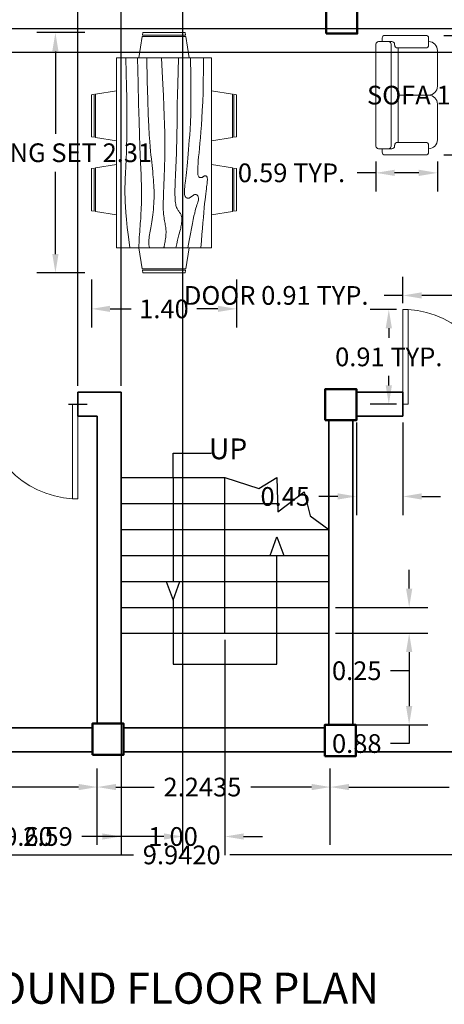
# Model space of a CAD drawing. Units: metres. Extents: x 473.2 to 488.6, y 701.8 to 717.3.
# Tile 2 of 4: x 479.3 to 483.4, y 701.8 to 711.3. Entities that reach past the tile are written whole.
import ezdxf

# ---------------------------------------------------------------- set-up
doc = ezdxf.new("R2010")
doc.units = ezdxf.units.M
doc.header["$PDMODE"] = 32
for name, color, linetype, lineweight in [('A-ANNO-DIMS', 2, 'Continuous', 18), ('A-ANNO-TEXT', 7, 'Continuous', 25), ('A-COLS', 7, 'Continuous', 50), ('A-DOOR', 3, 'Continuous', 18), ('A-FLOR-STRS', 7, 'Continuous', 25), ('A-FURN', 8, 'Continuous', 18), ('A-WALL', 7, 'Continuous', 35)]:
    doc.layers.add(name, color=color, linetype=linetype, lineweight=lineweight)
doc.styles.get("Standard").update_dxf_attribs({"font": 'arial.ttf'})
doc.dimstyles.get("Standard").update_dxf_attribs({"dimtxt": 0.18, "dimasz": 0.18, "dimexe": 0.18, "dimexo": 0.0625, "dimgap": 0.09, "dimtad": 0, "dimtih": 1, "dimtoh": 1, "dimdec": 4, "dimzin": 0, "dimdsep": 46, "dimtxsty": 'Standard', "dimcen": 0.09, "dimadec": 0, "dimazin": 0, "dimtfac": 1, "dimtdec": 4, "dimtofl": 0, "dimtmove": 0, "dimatfit": 3, "dimfxl": 1, "dimtolj": 1, "dimtzin": 0, "dimarcsym": 0})

# ---------------------------------------------------------------- blocks, each defined once
blk = doc.blocks.new('A$C02A636C4')
for p, q in [((1.203, 0.669), (0.097, 0.669)), ((0, 0.572), (0, 0.126)), ((0.068, 0.601), (0.029, 0.601)), ((0.068, 0.64), (0.068, 0.601)), ((0.068, 0.533), (0.068, 0.601)), ((0.068, 0.495), (0.068, 0.543)), ((1.232, 0.64), (1.232, 0.601)), ((1.232, 0.601), (1.271, 0.601)), ((1.232, 0.533), (1.232, 0.601)), ((1.232, 0.495), (1.232, 0.543)), ((1.3, 0.572), (1.3, 0.126)), ((1.203, 0.504), (0.097, 0.504)), ((0.107, 0.466), (0.097, 0.466)), ((0.136, 0.126), (0.136, 0.436)), ((1.164, 0.126), (1.164, 0.436)), ((1.193, 0.466), (1.203, 0.466)), ((1.164, 0.427), (0.136, 0.427)), ((0.65, 0.097), (0.65, 0.427)), ((0.029, 0.097), (0.107, 0.097)), ((0.165, 0), (0.553, 0)), ((0.747, 0), (1.135, 0)), ((1.271, 0.097), (1.193, 0.097))]:
    blk.add_line(p, q)
for centre, radius, start, end in [((0.097, 0.64), 0.0291, 90, 180), ((1.203, 0.64), 0.0291, 0, 90), ((0.029, 0.572), 0.0291, 90, 180), ((1.271, 0.572), 0.0291, 0, 90), ((0.097, 0.533), 0.0291, 180, 270), ((0.097, 0.495), 0.0291, 180, 270), ((0.107, 0.436), 0.0291, 0, 90), ((1.193, 0.436), 0.0291, 90, 180), ((1.203, 0.533), 0.0291, 270, 0), ((1.203, 0.495), 0.0291, 270, 0), ((0.029, 0.126), 0.0291, 180, 270), ((0.107, 0.126), 0.0291, 270, 0), ((1.193, 0.126), 0.0291, 180, 270), ((1.271, 0.126), 0.0291, 270, 0), ((0.165, 0.097), 0.097, 180, 270), ((0.553, 0.097), 0.097, 270, 0), ((0.747, 0.097), 0.097, 180, 270), ((1.135, 0.097), 0.097, 270, 0)]:
    blk.add_arc(centre, radius, start, end)
blk = doc.blocks.new('Dining Set - 36 x 72 in.')
for p, q in [((-22, 27.5), (-22.1562, 26.50042)), ((-5.8416, 26.5), (-22.1534, 26.5)), ((-22, 27.5), (-6, 27.5)), ((-5.8437, 26.49966), (-6, 27.5)), ((6, 27.5), (5.8438, 26.50042)), ((22.1584, 26.5), (5.8466, 26.5)), ((6, 27.5), (22, 27.5)), ((22.1563, 26.49966), (22, 27.5)), ((-22.2343, 26.00059), (-23.4847, 17.99762)), ((-22.2304, 26), (-5.7608, 26)), ((-4.5152, 17.99762), (-5.7655, 25.99926)), ((5.7657, 26.00059), (4.5153, 17.99762)), ((5.7696, 26), (22.2392, 26)), ((23.4848, 17.99762), (22.2345, 25.99926)), ((36, 18), (-36, 18)), ((-36, 18), (-36, -18)), ((36, -18), (36, 18)), ((-45.5, 8), (-44.5004, 8.15617)), ((-45.5, 8), (-45.5, -8)), ((-44.5, -8.15843), (-44.5, 8.15338)), ((-44.0006, 8.23428), (-35.9976, 9.48474)), ((-44, 8.23041), (-44, -8.23915)), ((44.0006, 8.23428), (35.9976, 9.48474)), ((44, 8.23041), (44, -8.23915)), ((44.5, -8.15843), (44.5, 8.15338)), ((45.5, 8), (44.5005, 8.15617)), ((45.5, 8), (45.5, -8)), ((-44.4997, -8.15631), (-45.5, -8)), ((-35.9976, -9.48476), (-43.9993, -8.2345)), ((35.9976, -9.48476), (43.9993, -8.2345)), ((44.4997, -8.15631), (45.5, -8)), ((-36, -18), (36, -18)), ((-22.2343, -26.0006), (-23.4847, -17.99762)), ((-4.5152, -17.99762), (-5.7655, -25.99928)), ((5.7657, -26.0006), (4.5153, -17.99762)), ((23.4848, -17.99762), (22.2345, -25.99928)), ((-22.2304, -26), (-5.7608, -26)), ((5.7696, -26), (22.2392, -26)), ((-22, -27.5), (-22.1562, -26.50044)), ((-5.8416, -26.5), (-22.1534, -26.5)), ((-22, -27.5), (-6, -27.5)), ((-5.8437, -26.49967), (-6, -27.5)), ((6, -27.5), (5.8438, -26.50044)), ((22.1584, -26.5), (5.8466, -26.5)), ((6, -27.5), (22, -27.5)), ((22.1563, -26.49967), (22, -27.5))]:
    blk.add_line(p, q)
for points in [[(-36, 15), (-31.1772, 14.97754), (-26.8079, 14.91406), (-22.8538, 14.81543), (-19.276, 14.6875), (-16.0362, 14.53613), (-13.0957, 14.36718), (-10.4159, 14.18652), (-7.9583, 14), (-5.6904, 13.81315), (-3.6035, 13.63021), (-1.6954, 13.45508), (0.0365, 13.29166), (1.5945, 13.14388), (2.9811, 13.01562), (4.1988, 12.9108), (5.25, 12.83333), (6.1393, 12.78613), (6.8802, 12.76823), (7.4883, 12.77767), (7.9792, 12.8125), (8.3685, 12.87077), (8.6719, 12.95052), (8.9049, 13.0498), (9.0833, 13.16666), (9.2205, 13.29899), (9.3216, 13.44401), (9.3895, 13.59879), (9.4271, 13.76041), (9.4373, 13.92594), (9.4232, 14.09245), (9.3875, 14.257), (9.3333, 14.41666), (9.2638, 14.56917), (9.1836, 14.71484), (9.0975, 14.85465), (9.0104, 14.98958), (8.9272, 15.1206), (8.8529, 15.2487), (8.7922, 15.37483), (8.75, 15.5), (8.7305, 15.62467), (8.7344, 15.74739), (8.7617, 15.86621), (8.8125, 15.97916), (8.8867, 16.08431), (8.9844, 16.17968), (9.1055, 16.26334), (9.25, 16.33333), (9.4189, 16.38802), (9.6172, 16.42708), (9.8506, 16.45052), (10.125, 16.45833), (10.4463, 16.45052), (10.8203, 16.42708), (11.2529, 16.38802), (11.75, 16.33333), (12.3184, 16.26318), (12.9694, 16.17838), (13.7151, 16.07991), (14.5677, 15.96875), (15.5395, 15.84586), (16.6426, 15.71224), (17.8893, 15.56884), (19.2917, 15.41666), (20.859, 15.25667), (22.5879, 15.08984), (24.4721, 14.91715), (26.5052, 14.73958), (28.6809, 14.5581), (30.9929, 14.3737), (33.4347, 14.18733), (36, 14)], [(-36, 10), (-28.9766, 10.14274), (-23.1725, 10.20442), (-18.4241, 10.19775), (-14.5677, 10.13541), (-11.4399, 10.03011), (-8.877, 9.89453), (-6.7154, 9.74137), (-4.7917, 9.58333), (-2.9698, 9.43082), (-1.2246, 9.28515), (0.4415, 9.14534), (2.026, 9.01041), (3.5266, 8.87939), (4.9408, 8.7513), (6.266, 8.62516), (7.5, 8.5), (8.6411, 8.37549), (9.6914, 8.2539), (10.6538, 8.13818), (11.5312, 8.03125), (12.3267, 7.93603), (13.043, 7.85547), (13.6831, 7.79248), (14.25, 7.75), (14.7471, 7.7303), (15.1797, 7.73307), (15.5537, 7.75732), (15.875, 7.80208), (16.1494, 7.86637), (16.3828, 7.94922), (16.5811, 8.04964), (16.75, 8.16666), (16.8944, 8.29915), (17.0143, 8.44531), (17.1089, 8.60319), (17.1771, 8.77083), (17.218, 8.94629), (17.2305, 9.1276), (17.2137, 9.31282), (17.1667, 9.5), (17.0895, 9.6875), (16.987, 9.875), (16.8649, 10.0625), (16.7292, 10.25), (16.5856, 10.4375), (16.4401, 10.625), (16.2985, 10.8125), (16.1667, 11), (16.05, 11.18733), (15.9518, 11.3737), (15.8752, 11.5581), (15.8229, 11.73958), (15.798, 11.91715), (15.8034, 12.08984), (15.842, 12.25667), (15.9167, 12.41666), (16.0295, 12.56836), (16.1784, 12.70833), (16.3605, 12.83268), (16.5729, 12.9375), (16.8127, 13.01888), (17.0768, 13.07291), (17.3625, 13.0957), (17.6667, 13.08333), (17.9894, 13.03312), (18.3418, 12.94726), (18.7382, 12.82918), (19.1927, 12.68229), (19.7195, 12.51001), (20.3327, 12.31575), (21.0465, 12.10294), (21.875, 11.875), (22.8357, 11.63354), (23.959, 11.37304), (25.2786, 11.08618), (26.8282, 10.76562), (28.6414, 10.40405), (30.752, 9.99414), (33.1936, 9.52856), (36, 9)], [(-36, 5.5), (-30.7157, 5.3348), (-26.069, 5.20963), (-21.9946, 5.11767), (-18.4271, 5.05208), (-15.3009, 5.00602), (-12.5508, 4.97265), (-10.1112, 4.94515), (-7.9167, 4.91666), (-5.909, 4.88167), (-4.0586, 4.83984), (-2.3429, 4.79215), (-0.7396, 4.73958), (0.7739, 4.6831), (2.22, 4.6237), (3.6213, 4.56233), (5, 4.5), (6.373, 4.43782), (7.7344, 4.3776), (9.0723, 4.32129), (10.375, 4.27083), (11.6309, 4.22819), (12.8281, 4.19531), (13.9551, 4.17415), (15, 4.16666), (15.954, 4.17448), (16.819, 4.19791), (17.6001, 4.23698), (18.3021, 4.29166), (18.9299, 4.36198), (19.4883, 4.44791), (19.9823, 4.54948), (20.4167, 4.66666), (20.7969, 4.79899), (21.1302, 4.94401), (21.4245, 5.09879), (21.6875, 5.26041), (21.9271, 5.42594), (22.1511, 5.59245), (22.3672, 5.757), (22.5834, 5.91666), (22.8065, 6.06868), (23.0404, 6.21093), (23.2879, 6.34147), (23.5521, 6.45833), (23.8358, 6.55957), (24.142, 6.64323), (24.4735, 6.70735), (24.8334, 6.75), (25.2235, 6.76969), (25.642, 6.76692), (26.0858, 6.74267), (26.5521, 6.69791), (27.0379, 6.63362), (27.5404, 6.55078), (28.0565, 6.45036), (28.5834, 6.33333), (29.1242, 6.19987), (29.7071, 6.04687), (30.3661, 5.87044), (31.1354, 5.66666), (32.0493, 5.43164), (33.142, 5.16146), (34.4475, 4.85221), (36, 4.5)], [(-36, -1), (-30.7915, -0.6591), (-26.0195, -0.38216), (-21.6519, -0.16284), (-17.6563, 0.00521), (-14.0005, 0.12833), (-10.6523, 0.21289), (-7.5796, 0.26522), (-4.75, 0.29166), (-2.134, 0.29793), (0.2878, 0.28711), (2.5317, 0.26163), (4.6146, 0.22396), (6.5529, 0.17651), (8.3633, 0.12174), (10.0623, 0.06209), (11.6667, 0), (13.1899, -0.06201), (14.6341, -0.1211), (15.9982, -0.17432), (17.2813, -0.21875), (18.4823, -0.25147), (19.6003, -0.26953), (20.6343, -0.27002), (21.5834, -0.25), (22.4481, -0.20768), (23.2357, -0.14584), (23.9549, -0.06836), (24.6146, 0.02083), (25.2235, 0.11784), (25.7904, 0.21875), (26.3241, 0.31966), (26.8334, 0.41666), (27.3265, 0.50618), (27.8099, 0.58593), (28.2894, 0.65397), (28.7709, 0.70833), (29.2601, 0.74707), (29.763, 0.76823), (30.2855, 0.76985), (30.8334, 0.75), (31.4088, 0.70784), (31.9994, 0.64713), (32.589, 0.57275), (33.1615, 0.48958), (33.7008, 0.4025), (34.1908, 0.3164), (34.6153, 0.23616), (34.9584, 0.16666), (35.2099, 0.11165), (35.3848, 0.07031), (35.504, 0.04069), (35.5886, 0.02083), (35.6594, 0.00879), (35.7377, 0.0026), (35.8442, 0.00032), (36, 0)], [(-36, -6.5), (-27.1843, -6.31267), (-20.084, -6.1263), (-14.469, -5.9419), (-10.1094, -5.76042), (-6.7752, -5.58285), (-4.2363, -5.41016), (-2.2629, -5.24333), (-0.625, -5.08334), (0.8708, -4.93099), (2.2715, -4.78646), (3.5872, -4.64974), (4.8281, -4.52084), (6.0046, -4.39974), (7.127, -4.28646), (8.2053, -4.18099), (9.25, -4.08334), (10.2705, -3.99382), (11.2734, -3.91407), (12.2647, -3.84603), (13.25, -3.79167), (14.2354, -3.75293), (15.2266, -3.73177), (16.2295, -3.73015), (17.25, -3.75), (18.2912, -3.79248), (19.3451, -3.85547), (20.4009, -3.93604), (21.4479, -4.03125), (22.4754, -4.13819), (23.4727, -4.25391), (24.4289, -4.37549), (25.3334, -4.5), (26.1785, -4.62492), (26.9694, -4.74935), (27.7145, -4.87281), (28.4219, -4.99479), (29.1, -5.11483), (29.7572, -5.23242), (30.4016, -5.34709), (31.0417, -5.45834), (31.6837, -5.56437), (32.3262, -5.65821), (32.9658, -5.73153), (33.599, -5.77604), (34.2224, -5.78345), (34.8327, -5.74545), (35.4264, -5.65373), (36, -5.5)], [(-36, -10), (-26.4022, -9.81299), (-18.4675, -9.62891), (-11.9839, -9.45069), (-6.7396, -9.28125), (-2.5226, -9.12354), (0.8789, -8.98047), (3.6769, -8.85498), (6.0833, -8.75), (8.2767, -8.66765), (10.3021, -8.60677), (12.1712, -8.56543), (13.8958, -8.54167), (15.4876, -8.53353), (16.9583, -8.53907), (18.3197, -8.55632), (19.5834, -8.58334), (20.7616, -8.61841), (21.8685, -8.66081), (22.9188, -8.71004), (23.9271, -8.76563), (24.9081, -8.82707), (25.8763, -8.89388), (26.8465, -8.96558), (27.8334, -9.04167), (28.8474, -9.12118), (29.8828, -9.20117), (30.93, -9.27824), (31.9792, -9.34896), (33.0205, -9.40991), (34.0443, -9.45768), (35.0407, -9.48885), (36, -9.5)], [(-36, -14.5), (-30.0881, -14.33513), (-25.0332, -14.21224), (-20.7312, -14.12647), (-17.0781, -14.07292), (-13.97, -14.04671), (-11.3027, -14.04297), (-8.9724, -14.05681), (-6.875, -14.08334), (-4.9224, -14.11833), (-3.0905, -14.16016), (-1.3709, -14.20785), (0.2448, -14.26042), (1.7647, -14.3169), (3.1973, -14.3763), (4.5507, -14.43767), (5.8333, -14.5), (7.0554, -14.5621), (8.235, -14.62175), (9.3922, -14.67652), (10.5469, -14.72396), (11.7192, -14.76164), (12.929, -14.78711), (14.1965, -14.79794), (15.5417, -14.79167), (16.9933, -14.76424), (18.6152, -14.70508), (20.4804, -14.60197), (22.6615, -14.44271), (25.2312, -14.21509), (28.2624, -13.9069), (31.8277, -13.50594), (36, -13)]]:
    blk.add_lwpolyline(points)
blk = doc.blocks.new('*D18')
at = {"layer": 'A-ANNO-DIMS', "color": 0, "lineweight": -2, "transparency": 16777216}
for p, q in [((475.798, 702.6656), (475.798, 703.4022)), ((485.74, 702.957), (485.74, 703.4022)), ((475.978, 703.2222), (480.3782, 703.2222)), ((485.56, 703.2222), (481.3049, 703.2222))]:
    blk.add_line(p, q, dxfattribs=at)
at = {"layer": 'A-ANNO-DIMS', "color": 0, "transparency": 16777216}
for points in [[(475.978, 703.2522), (475.978, 703.1922), (475.798, 703.2222)], [(485.56, 703.2522), (485.56, 703.1922), (485.74, 703.2222)]]:
    blk.add_solid(points, dxfattribs=at)
at = {"layer": 'Defpoints', "color": 0, "transparency": 16777216}
for p in [(485.74, 703.2222), (485.74, 702.8945), (475.798, 702.6031)]:
    blk.add_point(p, dxfattribs=at)
at = {"layer": 'A-ANNO-DIMS', "color": 0, "transparency": 16777216, "insert": (480.8416, 703.2222), "char_height": 0.18, "width": 1.240263, "attachment_point": 5}
blk.add_mtext('\\A1;9.9420', dxfattribs=at)
blk = doc.blocks.new('*D19')
at = {"layer": 'A-ANNO-DIMS', "color": 0, "lineweight": -2, "transparency": 16777216}
for p, q in [((475.798, 703.4647), (475.798, 704.0553)), ((480.028, 703.6173), (480.028, 704.0553)), ((475.978, 703.8753), (477.468, 703.8753)), ((479.848, 703.8753), (478.4019, 703.8753))]:
    blk.add_line(p, q, dxfattribs=at)
at = {"layer": 'A-ANNO-DIMS', "color": 0, "transparency": 16777216}
for points in [[(475.978, 703.9053), (475.978, 703.8453), (475.798, 703.8753)], [(479.848, 703.9053), (479.848, 703.8453), (480.028, 703.8753)]]:
    blk.add_solid(points, dxfattribs=at)
at = {"layer": 'Defpoints', "color": 0, "transparency": 16777216}
for p in [(480.028, 703.8753), (480.028, 703.5548), (475.798, 703.4022)]:
    blk.add_point(p, dxfattribs=at)
at = {"layer": 'A-ANNO-DIMS', "color": 0, "transparency": 16777216, "insert": (477.9349, 703.8753), "char_height": 0.18, "width": 1.240263, "attachment_point": 5}
blk.add_mtext('\\A1;4.2300', dxfattribs=at)
blk = doc.blocks.new('*D20')
at = {"layer": 'A-ANNO-DIMS', "color": 0, "lineweight": -2, "transparency": 16777216}
for p, q in [((480.028, 703.3187), (480.028, 704.0553)), ((482.2714, 703.601), (482.2714, 704.0553)), ((480.208, 703.8753), (480.5754, 703.8753)), ((482.0914, 703.8753), (481.507, 703.8753))]:
    blk.add_line(p, q, dxfattribs=at)
at = {"layer": 'A-ANNO-DIMS', "color": 0, "transparency": 16777216}
for points in [[(480.208, 703.9053), (480.208, 703.8453), (480.028, 703.8753)], [(482.0914, 703.9053), (482.0914, 703.8453), (482.2714, 703.8753)]]:
    blk.add_solid(points, dxfattribs=at)
at = {"layer": 'Defpoints', "color": 0, "transparency": 16777216}
for p in [(482.2714, 703.8753), (482.2714, 703.5385), (480.028, 703.2562)]:
    blk.add_point(p, dxfattribs=at)
at = {"layer": 'A-ANNO-DIMS', "color": 0, "transparency": 16777216, "insert": (481.0412, 703.8753), "char_height": 0.18, "width": 1.240263, "attachment_point": 5}
blk.add_mtext('\\A1;2.2435', dxfattribs=at)
blk = doc.blocks.new('*D21')
at = {"layer": 'A-ANNO-DIMS', "color": 0, "lineweight": -2, "transparency": 16777216}
for p, q in [((482.2714, 703.3187), (482.2714, 704.0553)), ((485.7234, 703.5853), (485.7234, 704.0553)), ((482.4514, 703.8753), (483.415, 703.8753)), ((485.5434, 703.8753), (484.3415, 703.8753))]:
    blk.add_line(p, q, dxfattribs=at)
at = {"layer": 'A-ANNO-DIMS', "color": 0, "transparency": 16777216}
for points in [[(482.4514, 703.9053), (482.4514, 703.8453), (482.2714, 703.8753)], [(485.5434, 703.9053), (485.5434, 703.8453), (485.7234, 703.8753)]]:
    blk.add_solid(points, dxfattribs=at)
at = {"layer": 'Defpoints', "color": 0, "transparency": 16777216}
for p in [(485.7234, 703.8753), (485.7234, 703.5228), (482.2714, 703.2562)]:
    blk.add_point(p, dxfattribs=at)
at = {"layer": 'A-ANNO-DIMS', "color": 0, "transparency": 16777216, "insert": (483.8782, 703.8753), "char_height": 0.18, "width": 1.240263, "attachment_point": 5}
blk.add_mtext('\\A1;3.4520', dxfattribs=at)
blk = doc.blocks.new('DOOR-SWING-910')
for p, q in [((0, 0), (-0.05, 0)), ((-0.05, 0), (-0.05, -0.91)), ((0, 0), (0, -0.91)), ((0, -0.91), (-0.05, -0.91))]:
    blk.add_line(p, q)
blk.add_arc((0.0015, 0), 0.9115, 180, 266.76381)
blk = doc.blocks.new('COL-SQUARE-300')
blk.add_lwpolyline([(-0.15, -0.15), (0.15, -0.15), (0.15, 0.15), (-0.15, 0.15)], close=True)
blk = doc.blocks.new('*D27')
at = {"layer": 'A-ANNO-DIMS', "color": 0, "lineweight": -2, "transparency": 16777216}
for p, q in [((482.9717, 708.5321), (482.9717, 708.7861)), ((483.8817, 708.5321), (483.8817, 708.7861)), ((482.9717, 708.6061), (482.7917, 708.6061)), ((483.7017, 708.6061), (483.1517, 708.6061))]:
    blk.add_line(p, q, dxfattribs=at)
at = {"layer": 'A-ANNO-DIMS', "color": 0, "transparency": 16777216}
for points in [[(483.1517, 708.6361), (483.1517, 708.5761), (482.9717, 708.6061)], [(483.7017, 708.6361), (483.7017, 708.5761), (483.8817, 708.6061)]]:
    blk.add_solid(points, dxfattribs=at)
at = {"layer": 'Defpoints', "color": 0, "transparency": 16777216}
for p in [(482.9717, 708.6061), (482.9717, 708.4696), (483.8817, 708.4696)]:
    blk.add_point(p, dxfattribs=at)
at = {"layer": 'A-ANNO-DIMS', "color": 0, "transparency": 16777216, "insert": (481.7511, 708.6061), "char_height": 0.18, "attachment_point": 5}
blk.add_mtext('\\A1;DOOR 0.91 TYP.', dxfattribs=at)
blk = doc.blocks.new('*D28')
at = {"layer": 'A-ANNO-DIMS', "color": 0, "lineweight": -2, "transparency": 16777216}
for p, q in [((482.9092, 708.4696), (482.6552, 708.4696)), ((482.8352, 708.2896), (482.8352, 708.1965)), ((482.8352, 707.7396), (482.8352, 707.8327)), ((482.9092, 707.5596), (482.6552, 707.5596))]:
    blk.add_line(p, q, dxfattribs=at)
at = {"layer": 'A-ANNO-DIMS', "color": 0, "transparency": 16777216}
for points in [[(482.8052, 708.2896), (482.8652, 708.2896), (482.8352, 708.4696)], [(482.8052, 707.7396), (482.8652, 707.7396), (482.8352, 707.5596)]]:
    blk.add_solid(points, dxfattribs=at)
at = {"layer": 'Defpoints', "color": 0, "transparency": 16777216}
for p in [(482.9717, 708.4696), (482.8352, 707.5596), (482.9717, 707.5596)]:
    blk.add_point(p, dxfattribs=at)
at = {"layer": 'A-ANNO-DIMS', "color": 0, "transparency": 16777216, "insert": (482.8352, 708.0146), "char_height": 0.18, "attachment_point": 5}
blk.add_mtext('\\A1;0.91 TYP.', dxfattribs=at)
blk = doc.blocks.new('*D33')
at = {"layer": 'A-ANNO-DIMS', "color": 0, "lineweight": -2, "transparency": 16777216}
for p, q in [((483.3662, 711.1086), (483.6562, 711.1086)), ((483.4762, 710.9286), (483.4762, 710.7165)), ((483.4762, 710.1382), (483.4762, 710.3503)), ((483.3662, 709.9582), (483.6562, 709.9582))]:
    blk.add_line(p, q, dxfattribs=at)
at = {"layer": 'A-ANNO-DIMS', "color": 0, "transparency": 16777216}
for points in [[(483.4462, 710.9286), (483.5062, 710.9286), (483.4762, 711.1086)], [(483.4462, 710.1382), (483.5062, 710.1382), (483.4762, 709.9582)]]:
    blk.add_solid(points, dxfattribs=at)
at = {"layer": 'Defpoints', "color": 0, "transparency": 16777216}
for p in [(483.3037, 711.1086), (483.3037, 709.9582), (483.4762, 709.9582)]:
    blk.add_point(p, dxfattribs=at)
at = {"layer": 'A-ANNO-DIMS', "color": 0, "transparency": 16777216, "insert": (483.4762, 710.5334), "char_height": 0.18, "attachment_point": 5}
blk.add_mtext('\\A1;SOFA 1.15 TYP.', dxfattribs=at)
blk = doc.blocks.new('*D34')
at = {"layer": 'A-ANNO-DIMS', "color": 0, "lineweight": -2, "transparency": 16777216}
for p, q in [((482.7113, 709.8957), (482.7113, 709.6057)), ((483.3037, 709.8957), (483.3037, 709.6057)), ((482.7113, 709.7857), (482.5313, 709.7857)), ((483.1237, 709.7857), (482.8913, 709.7857))]:
    blk.add_line(p, q, dxfattribs=at)
at = {"layer": 'A-ANNO-DIMS', "color": 0, "transparency": 16777216}
for points in [[(482.8913, 709.8157), (482.8913, 709.7557), (482.7113, 709.7857)], [(483.1237, 709.8157), (483.1237, 709.7557), (483.3037, 709.7857)]]:
    blk.add_solid(points, dxfattribs=at)
at = {"layer": 'Defpoints', "color": 0, "transparency": 16777216}
for p in [(482.7113, 709.9582), (483.3037, 709.9582), (482.7113, 709.7857)]:
    blk.add_point(p, dxfattribs=at)
at = {"layer": 'A-ANNO-DIMS', "color": 0, "transparency": 16777216, "insert": (481.8984, 709.7857), "char_height": 0.18, "attachment_point": 5}
blk.add_mtext('\\A1;0.59 TYP.', dxfattribs=at)
blk = doc.blocks.new('*D37')
at = {"layer": 'A-ANNO-DIMS', "color": 0, "lineweight": -2, "transparency": 16777216}
for p, q in [((479.9098, 711.1348), (479.4456, 711.1348)), ((479.6256, 710.9548), (479.6256, 710.1622)), ((479.6256, 709.0034), (479.6256, 709.796)), ((479.9098, 708.8234), (479.4456, 708.8234))]:
    blk.add_line(p, q, dxfattribs=at)
at = {"layer": 'A-ANNO-DIMS', "color": 0, "transparency": 16777216}
for points in [[(479.5956, 710.9548), (479.6556, 710.9548), (479.6256, 711.1348)], [(479.5956, 709.0034), (479.6556, 709.0034), (479.6256, 708.8234)]]:
    blk.add_solid(points, dxfattribs=at)
at = {"layer": 'Defpoints', "color": 0, "transparency": 16777216}
for p in [(479.9723, 711.1348), (479.6256, 708.8234), (479.9723, 708.8234)]:
    blk.add_point(p, dxfattribs=at)
at = {"layer": 'A-ANNO-DIMS', "color": 0, "transparency": 16777216, "insert": (479.6256, 709.9791), "char_height": 0.18, "attachment_point": 5}
blk.add_mtext('\\A1;DINING SET 2.31', dxfattribs=at)
blk = doc.blocks.new('*D38')
at = {"layer": 'A-ANNO-DIMS', "color": 0, "lineweight": -2, "transparency": 16777216}
for p, q in [((479.9723, 708.7609), (479.9723, 708.2967)), ((481.3693, 708.7609), (481.3693, 708.2967)), ((480.1523, 708.4767), (480.3558, 708.4767)), ((481.1893, 708.4767), (480.9858, 708.4767))]:
    blk.add_line(p, q, dxfattribs=at)
at = {"layer": 'A-ANNO-DIMS', "color": 0, "transparency": 16777216}
for points in [[(480.1523, 708.5067), (480.1523, 708.4467), (479.9723, 708.4767)], [(481.1893, 708.5067), (481.1893, 708.4467), (481.3693, 708.4767)]]:
    blk.add_solid(points, dxfattribs=at)
at = {"layer": 'Defpoints', "color": 0, "transparency": 16777216}
for p in [(479.9723, 708.8234), (481.3693, 708.8234), (481.3693, 708.4767)]:
    blk.add_point(p, dxfattribs=at)
at = {"layer": 'A-ANNO-DIMS', "color": 0, "transparency": 16777216, "insert": (480.6708, 708.4767), "char_height": 0.18, "attachment_point": 5}
blk.add_mtext('\\A1;1.40', dxfattribs=at)
blk = doc.blocks.new('*D44')
at = {"layer": 'A-ANNO-DIMS', "color": 0, "lineweight": -2, "transparency": 16777216}
for p, q in [((486.5158, 711.3546), (486.5158, 711.5346)), ((486.5158, 711.5346), (486.6958, 711.5346)), ((478.5905, 711.1746), (486.6958, 711.1746)), ((478.5905, 710.9478), (486.6958, 710.9478)), ((486.5158, 710.7678), (486.5158, 710.5878))]:
    blk.add_line(p, q, dxfattribs=at)
at = {"layer": 'A-ANNO-DIMS', "color": 0, "transparency": 16777216}
for points in [[(486.4858, 711.3546), (486.5458, 711.3546), (486.5158, 711.1746)], [(486.4858, 710.7678), (486.5458, 710.7678), (486.5158, 710.9478)]]:
    blk.add_solid(points, dxfattribs=at)
at = {"layer": 'Defpoints', "color": 0, "transparency": 16777216}
for p in [(478.528, 711.1746), (486.5158, 711.1746), (478.528, 710.9478)]:
    blk.add_point(p, dxfattribs=at)
at = {"layer": 'A-ANNO-DIMS', "color": 0, "transparency": 16777216, "insert": (487.0196, 711.5346), "char_height": 0.18, "attachment_point": 5}
blk.add_mtext('\\A1;0.23', dxfattribs=at)
blk = doc.blocks.new('*D49')
at = {"layer": 'A-ANNO-DIMS', "color": 0, "lineweight": -2, "transparency": 16777216}
for p, q in [((482.5231, 707.3821), (482.5231, 706.4916)), ((482.9717, 707.3821), (482.9717, 706.4916)), ((482.3431, 706.6716), (482.1631, 706.6716)), ((483.1517, 706.6716), (483.3317, 706.6716))]:
    blk.add_line(p, q, dxfattribs=at)
at = {"layer": 'A-ANNO-DIMS', "color": 0, "transparency": 16777216}
for points in [[(482.3431, 706.7016), (482.3431, 706.6416), (482.5231, 706.6716)], [(483.1517, 706.7016), (483.1517, 706.6416), (482.9717, 706.6716)]]:
    blk.add_solid(points, dxfattribs=at)
at = {"layer": 'Defpoints', "color": 0, "transparency": 16777216}
for p in [(482.5231, 707.4446), (482.9717, 707.4446), (482.5231, 706.6716)]:
    blk.add_point(p, dxfattribs=at)
at = {"layer": 'A-ANNO-DIMS', "color": 0, "transparency": 16777216, "insert": (481.8386, 706.6716), "char_height": 0.18, "attachment_point": 5}
blk.add_mtext('\\A1;0.45', dxfattribs=at)
blk = doc.blocks.new('*D50')
at = {"layer": 'A-ANNO-DIMS', "color": 0, "lineweight": -2, "transparency": 16777216}
for p, q in [((479.8413, 707.7371), (479.8413, 717.3427)), ((480.258, 707.7371), (480.258, 717.3427)), ((479.6613, 717.1627), (479.4813, 717.1627)), ((480.438, 717.1627), (480.618, 717.1627))]:
    blk.add_line(p, q, dxfattribs=at)
at = {"layer": 'A-ANNO-DIMS', "color": 0, "transparency": 16777216}
for points in [[(479.6613, 717.1927), (479.6613, 717.1327), (479.8413, 717.1627)], [(480.438, 717.1927), (480.438, 717.1327), (480.258, 717.1627)]]:
    blk.add_solid(points, dxfattribs=at)
at = {"layer": 'Defpoints', "color": 0, "transparency": 16777216}
for p in [(480.258, 717.1627), (479.8413, 707.6746), (480.258, 707.6746)]:
    blk.add_point(p, dxfattribs=at)
at = {"layer": 'A-ANNO-DIMS', "color": 0, "transparency": 16777216, "insert": (480.9408, 717.1627), "char_height": 0.18, "attachment_point": 5}
blk.add_mtext('\\A1;0.42', dxfattribs=at)
blk = doc.blocks.new('*D51')
at = {"layer": 'A-ANNO-DIMS', "color": 0, "lineweight": -2, "transparency": 16777216}
for p, q in [((480.257967, 705.292057), (480.257967, 703.219503)), ((481.257967, 705.292057), (481.257967, 703.219503)), ((480.077967, 703.399503), (479.897967, 703.399503)), ((481.437967, 703.399503), (481.617967, 703.399503))]:
    blk.add_line(p, q, dxfattribs=at)
at = {"layer": 'A-ANNO-DIMS', "color": 0, "transparency": 16777216}
for points in [[(480.077967, 703.429503), (480.077967, 703.369503), (480.257967, 703.399503)], [(481.437967, 703.429503), (481.437967, 703.369503), (481.257967, 703.399503)]]:
    blk.add_solid(points, dxfattribs=at)
at = {"layer": 'Defpoints', "color": 0, "transparency": 16777216}
for p in [(480.257967, 705.354557), (481.257967, 705.354557), (481.257967, 703.399503)]:
    blk.add_point(p, dxfattribs=at)
at = {"layer": 'A-ANNO-DIMS', "color": 0, "transparency": 16777216, "insert": (480.757967, 703.399503), "char_height": 0.18, "attachment_point": 5}
blk.add_mtext('\\A1;1.00', dxfattribs=at)
blk = doc.blocks.new('*D52')
at = {"layer": 'A-ANNO-DIMS', "color": 0, "lineweight": -2, "transparency": 16777216}
for p, q in [((483.031, 705.7846), (483.031, 705.9646)), ((482.3205, 705.6046), (483.211, 705.6046)), ((482.3205, 705.3546), (483.211, 705.3546)), ((483.031, 705.1746), (483.031, 704.9946)), ((483.031, 704.9946), (482.851, 704.9946))]:
    blk.add_line(p, q, dxfattribs=at)
at = {"layer": 'A-ANNO-DIMS', "color": 0, "transparency": 16777216}
for points in [[(483.001, 705.7846), (483.061, 705.7846), (483.031, 705.6046)], [(483.001, 705.1746), (483.061, 705.1746), (483.031, 705.3546)]]:
    blk.add_solid(points, dxfattribs=at)
at = {"layer": 'Defpoints', "color": 0, "transparency": 16777216}
for p in [(482.258, 705.6046), (482.258, 705.3546), (483.031, 705.3546)]:
    blk.add_point(p, dxfattribs=at)
at = {"layer": 'A-ANNO-DIMS', "color": 0, "transparency": 16777216, "insert": (482.5265, 704.9946), "char_height": 0.18, "attachment_point": 5}
blk.add_mtext('\\A1;0.25', dxfattribs=at)
blk = doc.blocks.new('*D53')
at = {"layer": 'A-ANNO-DIMS', "color": 0, "lineweight": -2, "transparency": 16777216}
for p, q in [((482.3205, 705.3546), (483.211, 705.3546)), ((483.031, 705.1746), (483.031, 704.6539)), ((482.3205, 704.4739), (483.211, 704.4739)), ((483.031, 704.4739), (483.031, 704.2939)), ((483.031, 704.2939), (482.851, 704.2939))]:
    blk.add_line(p, q, dxfattribs=at)
at = {"layer": 'A-ANNO-DIMS', "color": 0, "transparency": 16777216}
for points in [[(483.001, 705.1746), (483.061, 705.1746), (483.031, 705.3546)], [(483.001, 704.6539), (483.061, 704.6539), (483.031, 704.4739)]]:
    blk.add_solid(points, dxfattribs=at)
at = {"layer": 'Defpoints', "color": 0, "transparency": 16777216}
for p in [(482.258, 705.3546), (482.258, 704.4739), (483.031, 704.4739)]:
    blk.add_point(p, dxfattribs=at)
at = {"layer": 'A-ANNO-DIMS', "color": 0, "transparency": 16777216, "insert": (482.527, 704.2939), "char_height": 0.18, "attachment_point": 5}
blk.add_mtext('\\A1;0.88', dxfattribs=at)
blk = doc.blocks.new('*D64')
at = {"layer": 'A-ANNO-DIMS', "color": 0, "lineweight": -2, "transparency": 16777216}
for p, q in [((478.258, 715.4721), (478.258, 703.2195)), ((480.8495, 715.4721), (480.8495, 703.2195)), ((478.438, 703.3995), (479.2283, 703.3995)), ((480.6695, 703.3995), (479.8793, 703.3995))]:
    blk.add_line(p, q, dxfattribs=at)
at = {"layer": 'A-ANNO-DIMS', "color": 0, "transparency": 16777216}
for points in [[(478.438, 703.4295), (478.438, 703.3695), (478.258, 703.3995)], [(480.6695, 703.4295), (480.6695, 703.3695), (480.8495, 703.3995)]]:
    blk.add_solid(points, dxfattribs=at)
at = {"layer": 'Defpoints', "color": 0, "transparency": 16777216}
for p in [(478.258, 715.5346), (480.8495, 715.5346), (480.8495, 703.3995)]:
    blk.add_point(p, dxfattribs=at)
at = {"layer": 'A-ANNO-DIMS', "color": 0, "transparency": 16777216, "insert": (479.5538, 703.3995), "char_height": 0.18, "attachment_point": 5}
blk.add_mtext('\\A1;2.59', dxfattribs=at)
blk = doc.blocks.new('*D66')
at = {"layer": 'A-ANNO-DIMS', "color": 0, "lineweight": -2, "transparency": 16777216}
for p, q in [((478.258, 714.9046), (478.258, 703.2195)), ((478.858, 714.9046), (478.858, 703.2195)), ((478.438, 703.3995), (478.678, 703.3995)), ((478.858, 703.3995), (479.038, 703.3995))]:
    blk.add_line(p, q, dxfattribs=at)
at = {"layer": 'A-ANNO-DIMS', "color": 0, "transparency": 16777216}
for points in [[(478.438, 703.4295), (478.438, 703.3695), (478.258, 703.3995)], [(478.678, 703.4295), (478.678, 703.3695), (478.858, 703.3995)]]:
    blk.add_solid(points, dxfattribs=at)
at = {"layer": 'Defpoints', "color": 0, "transparency": 16777216}
for p in [(478.258, 714.9671), (478.858, 714.9671), (478.858, 703.3995)]:
    blk.add_point(p, dxfattribs=at)
at = {"layer": 'A-ANNO-DIMS', "color": 0, "transparency": 16777216, "insert": (479.3614, 703.3995), "char_height": 0.18, "attachment_point": 5}
blk.add_mtext('\\A1;0.60', dxfattribs=at)
blk = doc.blocks.new('*D68')
at = {"layer": 'A-ANNO-DIMS', "color": 0, "lineweight": -2, "transparency": 16777216}
for p, q in [((479.8428, 707.4696), (479.8428, 707.6496)), ((479.7528, 707.5596), (479.9328, 707.5596)), ((478.7822, 706.5586), (479.049, 706.8104)), ((478.6022, 706.5586), (478.7822, 706.5586))]:
    blk.add_line(p, q, dxfattribs=at)
at = {"layer": 'A-ANNO-DIMS', "color": 0, "transparency": 16777216}
blk.add_solid([(479.0284, 706.8322), (479.0696, 706.7886), (479.1799, 706.9339)], dxfattribs=at)
at = {"layer": 'Defpoints', "color": 0, "transparency": 16777216}
for p in [(479.8428, 707.5596), (479.1799, 706.9339)]:
    blk.add_point(p, dxfattribs=at)
at = {"layer": 'A-ANNO-DIMS', "color": 0, "transparency": 16777216, "insert": (478.0148, 706.5586), "char_height": 0.18, "attachment_point": 5}
blk.add_mtext('\\A1;2X R0.91', dxfattribs=at)

msp = doc.modelspace()

# ---------------------------------------------------------------- linework, layer by layer
at = {"layer": 'A-FLOR-STRS'}
for p, q in [((480.75797, 706.85456), (480.75797, 707.08891)), ((480.75797, 707.08891), (481.12954, 707.08891)), ((480.25797, 706.85456), (481.25797, 706.85456)), ((480.75797, 706.85456), (480.75797, 705.85456)), ((481.25797, 705.35456), (481.25797, 706.85456)), ((480.25797, 706.60456), (481.25797, 706.60456)), ((481.25797, 706.60456), (481.76381, 706.60456)), ((480.25797, 706.35456), (481.25797, 706.35456)), ((481.25797, 706.35456), (482.25797, 706.35456)), ((481.69218, 706.10456), (481.75797, 706.28209)), ((481.75797, 706.28209), (481.82375, 706.10456)), ((480.25797, 706.10456), (481.25797, 706.10456)), ((481.25797, 706.10456), (482.25797, 706.10456)), ((481.75797, 705.05874), (481.75797, 706.10456)), ((480.25797, 705.85456), (481.25797, 705.85456)), ((480.69218, 705.85258), (480.75797, 705.67505)), ((480.75797, 705.67505), (480.82375, 705.85258)), ((481.25797, 705.85456), (482.25797, 705.85456)), ((480.75797, 705.67505), (480.75797, 705.05874)), ((480.25797, 705.60456), (481.25797, 705.60456)), ((481.25797, 705.60456), (482.25797, 705.60456)), ((480.25797, 705.35456), (481.25797, 705.35456)), ((481.25797, 705.35456), (482.25797, 705.35456)), ((480.75797, 705.05874), (481.75797, 705.05874))]:
    msp.add_line(p, q, dxfattribs=at)
msp.add_lwpolyline([(481.25797, 706.85456), (481.58449, 706.74774), (481.75797, 706.85456), (481.76571, 706.52294), (482.02193, 706.71651), (482.07818, 706.48547), (482.25797, 706.35456)], dxfattribs=at)
at = {"layer": 'A-WALL'}
for p, q in [((479.84132, 707.67456), (479.84132, 707.44456)), ((479.84132, 707.67456), (480.25797, 707.67456)), ((480.25797, 704.48627), (480.25797, 707.67456)), ((482.52309, 707.67456), (482.97304, 707.67456)), ((482.97169, 707.44456), (482.97169, 707.67456)), ((479.84132, 707.44456), (480.02797, 707.44456)), ((480.02797, 704.48627), (480.02797, 707.44456)), ((482.25797, 704.47386), (482.25797, 707.40452)), ((482.48797, 704.47386), (482.48797, 707.40452)), ((482.52309, 707.44456), (482.97169, 707.44456)), ((476.02797, 704.44456), (479.98215, 704.44456)), ((480.28215, 704.44456), (482.21829, 704.44456)), ((476.06459, 704.21456), (479.98215, 704.21456)), ((480.28215, 704.21456), (482.21829, 704.21456)), ((482.51829, 704.21456), (485.43996, 704.21456))]:
    msp.add_line(p, q, dxfattribs=at)

# ---------------------------------------------------------------- block references
at = {"layer": 'A-COLS'}
for p in [(482.38113, 711.27646), (482.37309, 707.55452), (480.13215, 704.33627), (482.36829, 704.32386)]:
    msp.add_blockref('COL-SQUARE-300', p, dxfattribs=at)
at = {"layer": 'A-DOOR', "rotation": 180}
msp.add_blockref('DOOR-SWING-910', (482.97169, 707.55956), dxfattribs=at)
at = {"layer": 'A-DOOR'}
msp.add_blockref('DOOR-SWING-910', (479.84132, 707.55956), dxfattribs=at)
at = {"layer": 'A-FURN'}
for name, p, xscale, yscale, zscale, rotation in [('Dining Set - 36 x 72 in.', (480.67083, 709.97912), 0.0254, 0.0254, 0.0254, 270), ('A$C02A636C4', (483.30365, 711.10856), -0.8851373679523337, 0.8851373679523337, 0.8851373679523337, 90)]:
    msp.add_blockref(name, p, dxfattribs=dict(at, xscale=xscale, yscale=yscale, zscale=zscale, rotation=rotation))

# ---------------------------------------------------------------- texts
at = {"layer": 'A-ANNO-TEXT', "attachment_point": 1}
for s, width, heights, insert, char_height in [('UP', 2.8211562, [0], (481.10314, 707.22989), 0.2), ('GROUND FLOOR PLAN', 7.0056545, [0.69309], (478.49827, 702.09007), 0.3)]:
    msp.add_mtext_dynamic_manual_height_columns(s, width=width, gutter_width=12.5, heights=heights, dxfattribs=dict(at, insert=insert, char_height=char_height))

# ---------------------------------------------------------------- dimensions: what is measured, and where the dimension line sits
at = {"layer": 'A-ANNO-DIMS'}
for base, p1, p2, picture, middle in [((480.25797, 717.16268), (479.84132, 707.67456), (480.25797, 707.67456), '*D50', (480.94083, 717.16268)), ((480.84954, 703.3995), (478.25797, 715.53456), (480.84954, 715.53456), '*D64', (479.55376, 703.3995)), ((478.85797, 703.3995), (478.25797, 714.9671), (478.85797, 714.9671), '*D66', (479.36144, 703.3995)), ((481.36933, 708.47671), (479.97233, 708.82342), (481.36933, 708.82342), '*D38', (480.67083, 708.47671)), ((481.25797, 703.3995), (480.25797, 705.35456), (481.25797, 705.35456), '*D51', (480.75797, 703.3995))]:
    dim = msp.add_linear_dim(base=base, p1=p1, p2=p2, dimstyle='Standard', override={"dimdec": 2, "dimlfac": 1, "dimrnd": 0, "dimzin": 0, "dimdsep": 46, "dimlunit": 2}, dxfattribs=at)
    dim.commit()
    dim.dimension.update_dxf_attribs({"geometry": picture, "text_midpoint": middle})
for base, p1, p2, angle, picture, middle in [((486.51584, 711.17456), (478.52797, 710.94776), (478.52797, 711.17456), 90, '*D44', (487.01962, 711.53456)), ((482.52309, 706.67156), (482.97169, 707.44456), (482.52309, 707.44456), 180, '*D49', (481.83864, 706.67156)), ((483.03097, 705.35456), (482.25797, 705.60456), (482.25797, 705.35456), 270, '*D52', (482.52651, 704.99456)), ((483.03097, 704.47387), (482.25797, 705.35456), (482.25797, 704.47387), 270, '*D53', (482.527, 704.29386))]:
    dim = msp.add_linear_dim(base=base, p1=p1, p2=p2, angle=angle, dimstyle='Standard', override={"dimdec": 2, "dimlfac": 1, "dimrnd": 0, "dimzin": 0, "dimdsep": 46, "dimlunit": 2}, dxfattribs=at)
    dim.commit()
    dim.dimension.update_dxf_attribs({"geometry": picture, "text_midpoint": middle})
for base, p1, p2, angle, text, picture, middle in [((479.62562, 708.82342), (479.97233, 711.13482), (479.97233, 708.82342), 270, 'DINING SET <>', '*D37', (479.62562, 709.97912)), ((483.4762, 709.95822), (483.30365, 711.10856), (483.30365, 709.95822), 270, 'SOFA <> TYP.', '*D33', (483.4762, 710.53339)), ((482.71131, 709.78567), (483.30365, 709.95822), (482.71131, 709.95822), 180, '<> TYP.', '*D34', (481.89836, 709.78567)), ((482.97169, 708.60606), (483.88169, 708.46956), (482.97169, 708.46956), 180, 'DOOR <> TYP.', '*D27', (481.7511, 708.60606)), ((482.83519, 707.55956), (482.97169, 708.46956), (482.97169, 707.55956), 270, '<> TYP.', '*D28', (482.83519, 708.01456))]:
    dim = msp.add_linear_dim(base=base, p1=p1, p2=p2, angle=angle, text=text, dimstyle='Standard', override={"dimdec": 2, "dimlfac": 1, "dimrnd": 0, "dimzin": 0, "dimdsep": 46, "dimlunit": 2}, dxfattribs=at)
    dim.commit()
    dim.dimension.update_dxf_attribs({"geometry": picture, "text_midpoint": middle})
dim = msp.add_radius_dim(center=(479.84277, 707.55956), mpoint=(479.17994, 706.93394), text='2X <>', dimstyle='Standard', override={"dimdec": 2, "dimlfac": 1, "dimrnd": 0, "dimzin": 0, "dimdsep": 46, "dimlunit": 2}, dxfattribs=at)
dim.commit()
dim.dimension.update_dxf_attribs({"geometry": '*D68', "text_midpoint": (478.01478, 706.55857), "dimtype": 164})
for base, p1, p2, picture, middle in [((480.02797, 703.87534), (475.79797, 703.40224), (480.02797, 703.55481), '*D19', (477.93495, 703.87534)), ((482.271425, 703.87534), (480.027967, 703.256193), (482.271425, 703.538545), '*D20', (481.041204, 703.87534)), ((485.72339, 703.87534), (482.27142, 703.25619), (485.72339, 703.52275), '*D21', (483.87823, 703.87534)), ((485.73996, 703.22224), (475.79797, 702.6031), (485.73996, 702.8945), '*D18', (480.84155, 703.22224))]:
    dim = msp.add_linear_dim(base=base, p1=p1, p2=p2, dimstyle='Standard', override={"dimclrd": 0, "dimclre": 0, "dimclrt": 0}, dxfattribs=at)
    dim.commit()
    dim.dimension.update_dxf_attribs({"geometry": picture, "text_midpoint": middle, "dimtype": 160})

doc.saveas('drawing.dxf')
